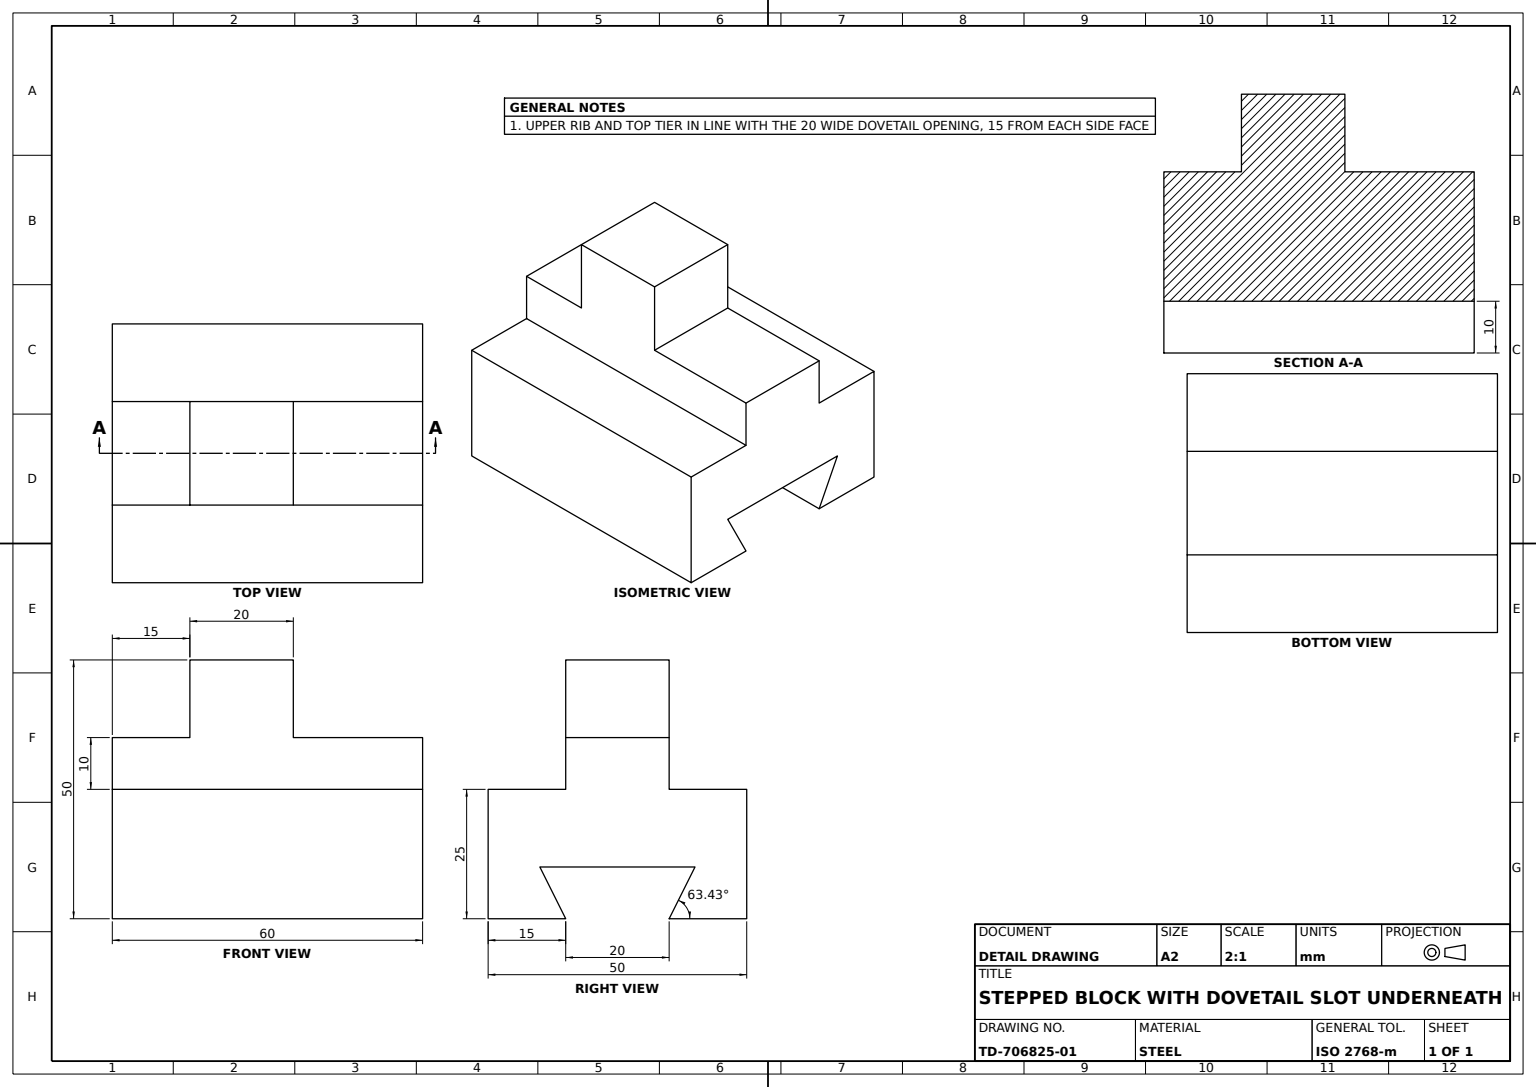
from build123d import *

# Parameters (mm, degrees)
STEPPED_BLOCK_60MM_DEPTH             = 30
UNDERSIDE_DOVETAIL_GROOVE_REACH      = 70.007
UNDERSIDE_DOVETAIL_GROOVE_SKETCH_W   = 15
UNDERSIDE_DOVETAIL_GROOVE_SKETCH_H   = 15
UNDERSIDE_DOVETAIL_GROOVE_SKETCH_W_2 = 25
TOP_TIER_POCKET_30X20_REACH          = 84.006


with BuildPart() as part:
    # Stepped Block Profile Sketch → Stepped Block 60mm (new, symmetric)
    with BuildSketch(Plane(origin=(0, 0, 0), x_dir=(0, 0, -1), z_dir=(1, 0, 0))):
        Polygon((-25, 0), (25, 0), (25, 25), (10, 25), (10, 50), (-10, 50), (-10, 25), (-25, 25), align=None)
    extrude(amount=STEPPED_BLOCK_60MM_DEPTH, both=True)

    # Underside Dovetail Groove Sketch → Underside Dovetail Groove (cut, up to next)
    with BuildSketch(Plane.XY.offset(10), mode=Mode.PRIVATE) as underside_dovetail_groove_sk1:
        with Locations((-22.5, 42.5)):
            Rectangle(UNDERSIDE_DOVETAIL_GROOVE_SKETCH_W, UNDERSIDE_DOVETAIL_GROOVE_SKETCH_H)
    underside_dovetail_groove_tool1 = extrude(underside_dovetail_groove_sk1.sketch, amount=-UNDERSIDE_DOVETAIL_GROOVE_REACH, mode=Mode.PRIVATE) & part.part
    # Underside Dovetail Groove Sketch → Underside Dovetail Groove (cut, up to next)
    with BuildSketch(Plane.XY.offset(10), mode=Mode.PRIVATE) as underside_dovetail_groove_sk2:
        with Locations((17.5, 42.5)):
            Rectangle(UNDERSIDE_DOVETAIL_GROOVE_SKETCH_W_2, UNDERSIDE_DOVETAIL_GROOVE_SKETCH_H)
    underside_dovetail_groove_tool2 = extrude(underside_dovetail_groove_sk2.sketch, amount=-UNDERSIDE_DOVETAIL_GROOVE_REACH, mode=Mode.PRIVATE) & part.part
    add(underside_dovetail_groove_tool1.solids().sort_by_distance((-22.5, 42.5, 10))[0], mode=Mode.SUBTRACT)
    add(underside_dovetail_groove_tool2.solids().sort_by_distance((17.5, 42.5, 10))[0], mode=Mode.SUBTRACT)

    # Top Tier Pocket Sketch → Top Tier Pocket 30x20 (cut, up to next)
    with BuildSketch(Plane(origin=(30, 0, 0), x_dir=(0, 0, -1), z_dir=(1, 0, 0)), mode=Mode.PRIVATE) as top_tier_pocket_30x20_sk1:
        Polygon((-10, 0), (-15, 10), (15, 10), (10, 0), align=None)
    top_tier_pocket_30x20_tool1 = extrude(top_tier_pocket_30x20_sk1.sketch, amount=-TOP_TIER_POCKET_30X20_REACH, mode=Mode.PRIVATE) & part.part
    add(top_tier_pocket_30x20_tool1.solids().sort_by_distance((30, 5.333333, 0))[0], mode=Mode.SUBTRACT)


solid = part.part
